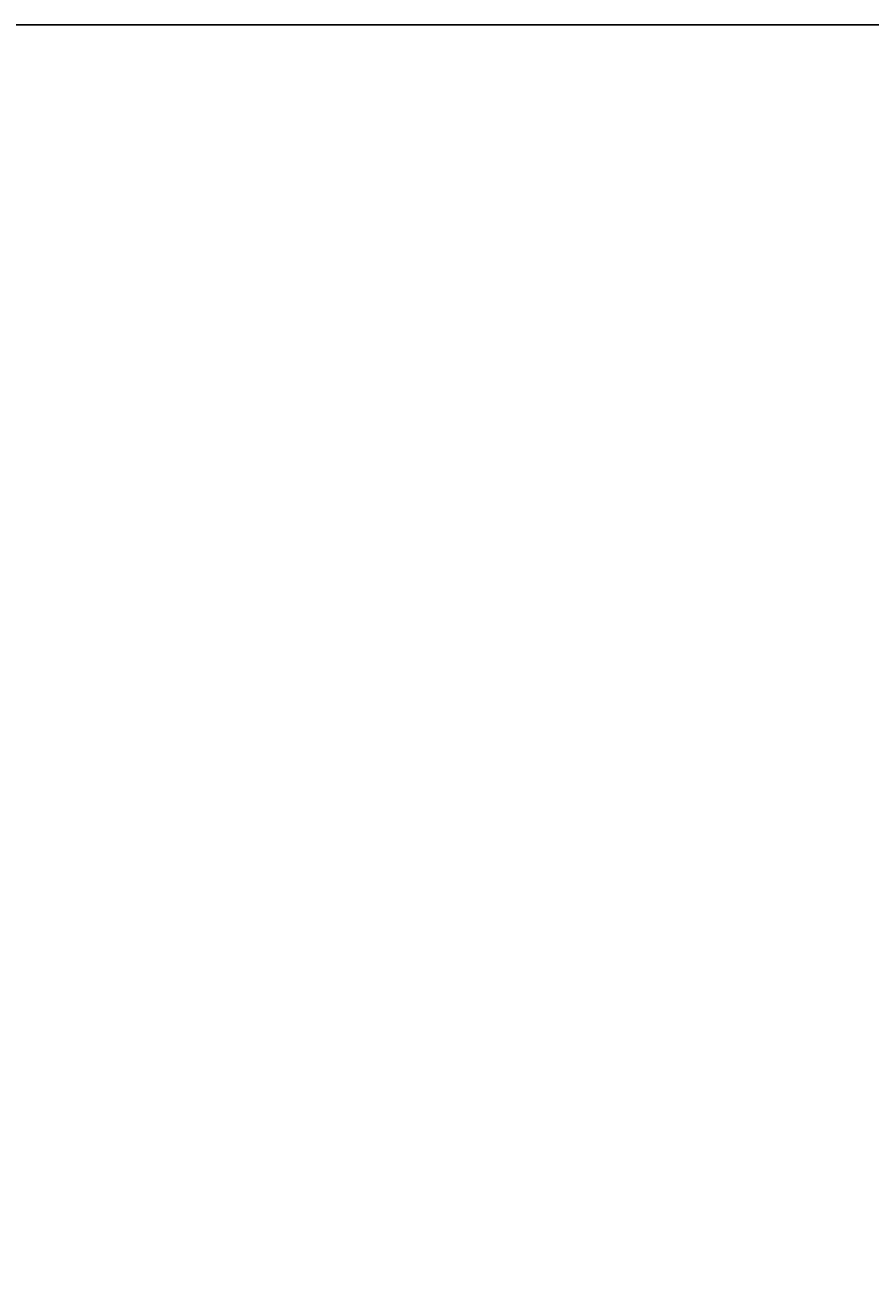
# Model space of a CAD drawing. Units: inches. Extents: x -61 to 1599, y -1316 to 257.
# Tile 28 of 204: x 416 to 442, y -912 to -873. Entities that reach past the tile are written whole.
import ezdxf

# ---------------------------------------------------------------- set-up
doc = ezdxf.new("R2010")
doc.units = ezdxf.units.IN
doc.header["$MEASUREMENT"] = 0
doc.layers.add('A-ANNO-DIMS', color=2, linetype='Continuous', lineweight=18)
doc.styles.get("Standard").update_dxf_attribs({"font": 'arial.ttf'})
doc.dimstyles.get("Standard").update_dxf_attribs({"dimtxt": 0.18, "dimasz": 0.18, "dimexe": 0.18, "dimexo": 0.0625, "dimgap": 0.09, "dimtad": 0, "dimtih": 1, "dimtoh": 1, "dimdec": 0, "dimzin": 0, "dimdsep": 46, "dimlunit": 3, "dimtxsty": 'Standard', "dimcen": 0.09, "dimadec": 0, "dimazin": 0, "dimtfac": 1, "dimtdec": 0, "dimtofl": 0, "dimtmove": 0, "dimatfit": 3, "dimfxl": 1, "dimtolj": 1, "dimtzin": 0, "dimarcsym": 0})

# ---------------------------------------------------------------- blocks, each defined once
blk = doc.blocks.new('*D696')
at = {"layer": 'A-ANNO-DIMS', "color": 0, "lineweight": -2, "transparency": 16777216}
for p, q in [((690.64, -873.169), (-61.077, -873.169)), ((-60.897, -873.349), (-60.897, -1025.799)), ((-60.897, -1178.613), (-60.897, -1026.163)), ((690.64, -1178.793), (-61.077, -1178.793))]:
    blk.add_line(p, q, dxfattribs=at)
at = {"layer": 'A-ANNO-DIMS', "color": 0, "transparency": 16777216}
for points in [[(-60.927, -873.349), (-60.867, -873.349), (-60.897, -873.169)], [(-60.927, -1178.613), (-60.867, -1178.613), (-60.897, -1178.793)]]:
    blk.add_solid(points, dxfattribs=at)
at = {"layer": 'DEFPOINTS', "color": 0, "transparency": 16777216}
for p in [(-60.897, -873.169), (690.703, -873.169), (690.703, -1178.793)]:
    blk.add_point(p, dxfattribs=at)
at = {"layer": 'A-ANNO-DIMS', "color": 0, "transparency": 16777216, "insert": (-60.897, -1025.981), "char_height": 0.18, "attachment_point": 5}
blk.add_mtext('\\A1;305.6', dxfattribs=at)

msp = doc.modelspace()

# ---------------------------------------------------------------- dimensions: what is measured, and where the dimension line sits
at = {"layer": 'A-ANNO-DIMS'}
dim = msp.add_linear_dim(base=(-60.8972, -873.169), p1=(690.7028, -1178.7933), p2=(690.7028, -873.169), angle=90, dimstyle='Standard', override={"dimdec": 1, "dimlfac": 1, "dimrnd": 0, "dimzin": 0, "dimdsep": 46, "dimlunit": 2}, dxfattribs=at)
dim.commit()
dim.dimension.update_dxf_attribs({"geometry": '*D696', "text_midpoint": (-60.8972, -1025.9812)})

doc.saveas('drawing.dxf')
